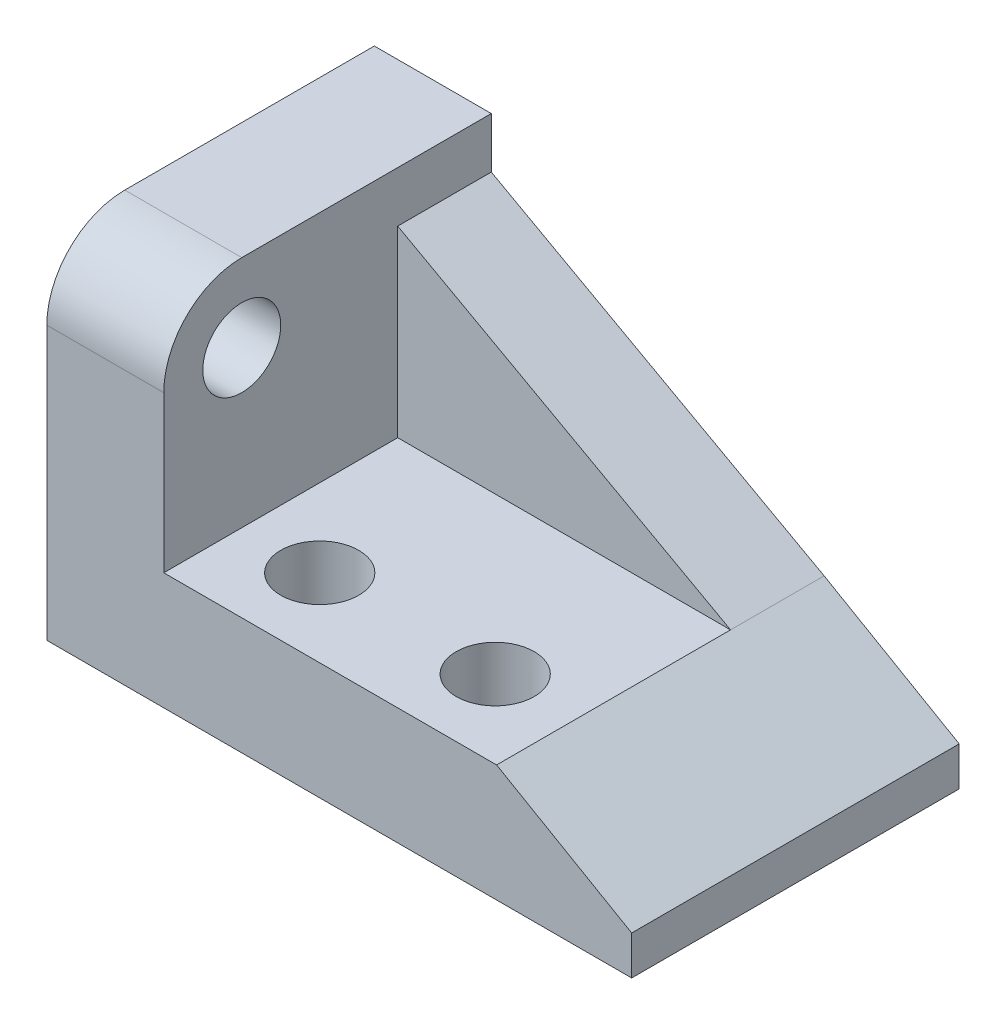
ISO-10303-21;
HEADER;
FILE_DESCRIPTION(('STEP AP214'),'2;1');
FILE_NAME('part.step','',(''),(''),'','','');
FILE_SCHEMA(('AUTOMOTIVE_DESIGN { 1 0 10303 214 1 1 1 1 }'));
ENDSEC;
DATA;
#1=APPLICATION_CONTEXT('core data for automotive mechanical design processes');
#2=APPLICATION_PROTOCOL_DEFINITION('international standard','automotive_design',2000,#1);
#3=PRODUCT_CONTEXT('',#1,'mechanical');
#4=PRODUCT('Part','Part','',(#3));
#5=PRODUCT_RELATED_PRODUCT_CATEGORY('part','',(#4));
#6=PRODUCT_DEFINITION_FORMATION('','',#4);
#7=PRODUCT_DEFINITION_CONTEXT('part definition',#1,'design');
#8=PRODUCT_DEFINITION('design','',#6,#7);
#9=PRODUCT_DEFINITION_SHAPE('','',#8);
#10=(LENGTH_UNIT() NAMED_UNIT(*) SI_UNIT(.MILLI.,.METRE.));
#11=(NAMED_UNIT(*) PLANE_ANGLE_UNIT() SI_UNIT($,.RADIAN.));
#12=(NAMED_UNIT(*) SI_UNIT($,.STERADIAN.) SOLID_ANGLE_UNIT());
#13=UNCERTAINTY_MEASURE_WITH_UNIT(LENGTH_MEASURE(1.E-05),#10,'distance_accuracy_value','');
#14=(GEOMETRIC_REPRESENTATION_CONTEXT(3) GLOBAL_UNCERTAINTY_ASSIGNED_CONTEXT((#13)) GLOBAL_UNIT_ASSIGNED_CONTEXT((#10,
#11,#12)) REPRESENTATION_CONTEXT('',''));
#15=CARTESIAN_POINT('',(0.,0.,0.));
#16=DIRECTION('',(0.,0.,1.));
#17=DIRECTION('',(1.,0.,0.));
#18=AXIS2_PLACEMENT_3D('',#15,#16,#17);
#19=CARTESIAN_POINT('',(40.3589838486223,30.,42.));
#20=DIRECTION('',(0.,-1.,0.));
#21=DIRECTION('',(1.,0.,0.));
#22=AXIS2_PLACEMENT_3D('',#19,#20,#21);
#23=PLANE('',#22);
#24=CARTESIAN_POINT('',(-25.,30.,22.));
#25=DIRECTION('',(0.,1.,0.));
#26=DIRECTION('',(-1.,0.,0.));
#27=AXIS2_PLACEMENT_3D('',#24,#25,#26);
#28=CIRCLE('',#27,10.);
#29=CARTESIAN_POINT('',(-35.,30.,22.));
#30=VERTEX_POINT('',#29);
#31=EDGE_CURVE('E214',#30,#30,#28,.T.);
#32=ORIENTED_EDGE('',*,*,#31,.F.);
#33=EDGE_LOOP('',(#32));
#34=FACE_BOUND('',#33,.T.);
#35=CARTESIAN_POINT('',(20.,30.,22.));
#36=DIRECTION('',(0.,1.,0.));
#37=DIRECTION('',(-1.,0.,0.));
#38=AXIS2_PLACEMENT_3D('',#35,#36,#37);
#39=CIRCLE('',#38,10.);
#40=CARTESIAN_POINT('',(9.99999999999999,30.,22.));
#41=VERTEX_POINT('',#40);
#42=EDGE_CURVE('E264',#41,#41,#39,.T.);
#43=ORIENTED_EDGE('',*,*,#42,.F.);
#44=EDGE_LOOP('',(#43));
#45=FACE_BOUND('',#44,.T.);
#46=DIRECTION('',(1.,0.,0.));
#47=VECTOR('',#46,1.);
#48=CARTESIAN_POINT('',(40.3589838486223,30.,-18.));
#49=LINE('',#48,#47);
#50=CARTESIAN_POINT('',(-45.,30.,-18.));
#51=VERTEX_POINT('',#50);
#52=CARTESIAN_POINT('',(40.3589838486223,30.,-18.));
#53=VERTEX_POINT('',#52);
#54=EDGE_CURVE('E153',#51,#53,#49,.T.);
#55=ORIENTED_EDGE('',*,*,#54,.F.);
#56=DIRECTION('',(0.,0.,-1.));
#57=VECTOR('',#56,1.);
#58=CARTESIAN_POINT('',(-45.,30.,42.));
#59=LINE('',#58,#57);
#60=CARTESIAN_POINT('',(-45.,30.,42.));
#61=VERTEX_POINT('',#60);
#62=EDGE_CURVE('E164',#61,#51,#59,.T.);
#63=ORIENTED_EDGE('',*,*,#62,.F.);
#64=DIRECTION('',(-1.,0.,0.));
#65=VECTOR('',#64,1.);
#66=CARTESIAN_POINT('',(40.3589838486223,30.,42.));
#67=LINE('',#66,#65);
#68=CARTESIAN_POINT('',(40.3589838486223,30.,42.));
#69=VERTEX_POINT('',#68);
#70=EDGE_CURVE('E144',#69,#61,#67,.T.);
#71=ORIENTED_EDGE('',*,*,#70,.F.);
#72=DIRECTION('',(0.,0.,-1.));
#73=VECTOR('',#72,1.);
#74=CARTESIAN_POINT('',(40.3589838486223,30.,42.));
#75=LINE('',#74,#73);
#76=EDGE_CURVE('E170',#69,#53,#75,.T.);
#77=ORIENTED_EDGE('',*,*,#76,.T.);
#78=EDGE_LOOP('',(#55,#63,#71,#77));
#79=FACE_BOUND('',#78,.T.);
#80=ADVANCED_FACE('F39',(#34,#45,#79),#23,.F.);
#81=CARTESIAN_POINT('',(-45.,90.,42.));
#82=DIRECTION('',(0.,-1.,0.));
#83=DIRECTION('',(0.,0.,-1.));
#84=AXIS2_PLACEMENT_3D('',#81,#82,#83);
#85=PLANE('',#84);
#86=DIRECTION('',(-1.,0.,0.));
#87=VECTOR('',#86,1.);
#88=CARTESIAN_POINT('',(-45.,90.,-42.));
#89=LINE('',#88,#87);
#90=CARTESIAN_POINT('',(-45.,90.,-42.));
#91=VERTEX_POINT('',#90);
#92=CARTESIAN_POINT('',(-75.,90.,-42.));
#93=VERTEX_POINT('',#92);
#94=EDGE_CURVE('E147',#91,#93,#89,.T.);
#95=ORIENTED_EDGE('',*,*,#94,.T.);
#96=DIRECTION('',(0.,0.,-1.));
#97=VECTOR('',#96,1.);
#98=CARTESIAN_POINT('',(-75.,90.,42.));
#99=LINE('',#98,#97);
#100=CARTESIAN_POINT('',(-75.,90.,22.));
#101=VERTEX_POINT('',#100);
#102=EDGE_CURVE('E135',#101,#93,#99,.T.);
#103=ORIENTED_EDGE('',*,*,#102,.F.);
#104=DIRECTION('',(-1.,0.,0.));
#105=VECTOR('',#104,1.);
#106=CARTESIAN_POINT('',(-45.,90.,22.));
#107=LINE('',#106,#105);
#108=CARTESIAN_POINT('',(-45.,90.,22.));
#109=VERTEX_POINT('',#108);
#110=EDGE_CURVE('E177',#101,#109,#107,.F.);
#111=ORIENTED_EDGE('',*,*,#110,.T.);
#112=DIRECTION('',(0.,0.,-1.));
#113=VECTOR('',#112,1.);
#114=CARTESIAN_POINT('',(-45.,90.,42.));
#115=LINE('',#114,#113);
#116=EDGE_CURVE('E149',#109,#91,#115,.T.);
#117=ORIENTED_EDGE('',*,*,#116,.T.);
#118=EDGE_LOOP('',(#95,#103,#111,#117));
#119=FACE_BOUND('',#118,.T.);
#120=ADVANCED_FACE('F189',(#119),#85,.F.);
#121=CARTESIAN_POINT('',(-75.,90.,42.));
#122=DIRECTION('',(1.,0.,0.));
#123=DIRECTION('',(0.,1.,0.));
#124=AXIS2_PLACEMENT_3D('',#121,#122,#123);
#125=PLANE('',#124);
#126=CARTESIAN_POINT('',(-75.,70.,22.));
#127=DIRECTION('',(1.,0.,0.));
#128=DIRECTION('',(0.,1.,0.));
#129=AXIS2_PLACEMENT_3D('',#126,#127,#128);
#130=CIRCLE('',#129,10.);
#131=CARTESIAN_POINT('',(-75.,80.,22.));
#132=VERTEX_POINT('',#131);
#133=EDGE_CURVE('E259',#132,#132,#130,.F.);
#134=ORIENTED_EDGE('',*,*,#133,.F.);
#135=EDGE_LOOP('',(#134));
#136=FACE_BOUND('',#135,.T.);
#137=DIRECTION('',(0.,-1.,0.));
#138=VECTOR('',#137,1.);
#139=CARTESIAN_POINT('',(-75.,90.,-42.));
#140=LINE('',#139,#138);
#141=CARTESIAN_POINT('',(-75.,0.,-42.));
#142=VERTEX_POINT('',#141);
#143=EDGE_CURVE('E129',#93,#142,#140,.T.);
#144=ORIENTED_EDGE('',*,*,#143,.T.);
#145=DIRECTION('',(0.,0.,-1.));
#146=VECTOR('',#145,1.);
#147=CARTESIAN_POINT('',(-75.,0.,42.));
#148=LINE('',#147,#146);
#149=CARTESIAN_POINT('',(-75.,0.,42.));
#150=VERTEX_POINT('',#149);
#151=EDGE_CURVE('E127',#150,#142,#148,.T.);
#152=ORIENTED_EDGE('',*,*,#151,.F.);
#153=DIRECTION('',(0.,-1.,0.));
#154=VECTOR('',#153,1.);
#155=CARTESIAN_POINT('',(-75.,90.,42.));
#156=LINE('',#155,#154);
#157=CARTESIAN_POINT('',(-75.,70.,42.));
#158=VERTEX_POINT('',#157);
#159=EDGE_CURVE('E114',#158,#150,#156,.T.);
#160=ORIENTED_EDGE('',*,*,#159,.F.);
#161=CARTESIAN_POINT('',(-75.,70.,22.));
#162=DIRECTION('',(1.,0.,0.));
#163=DIRECTION('',(0.,1.,0.));
#164=AXIS2_PLACEMENT_3D('',#161,#162,#163);
#165=CIRCLE('',#164,20.);
#166=EDGE_CURVE('E171',#158,#101,#165,.F.);
#167=ORIENTED_EDGE('',*,*,#166,.T.);
#168=ORIENTED_EDGE('',*,*,#102,.T.);
#169=EDGE_LOOP('',(#144,#152,#160,#167,#168));
#170=FACE_BOUND('',#169,.T.);
#171=ADVANCED_FACE('F130',(#136,#170),#125,.F.);
#172=CARTESIAN_POINT('',(-75.,0.,42.));
#173=DIRECTION('',(0.,1.,0.));
#174=DIRECTION('',(0.,0.,1.));
#175=AXIS2_PLACEMENT_3D('',#172,#173,#174);
#176=PLANE('',#175);
#177=CARTESIAN_POINT('',(-25.,0.,22.));
#178=DIRECTION('',(0.,1.,0.));
#179=DIRECTION('',(0.,0.,1.));
#180=AXIS2_PLACEMENT_3D('',#177,#178,#179);
#181=CIRCLE('',#180,10.);
#182=CARTESIAN_POINT('',(-25.,0.,32.));
#183=VERTEX_POINT('',#182);
#184=EDGE_CURVE('E207',#183,#183,#181,.F.);
#185=ORIENTED_EDGE('',*,*,#184,.F.);
#186=EDGE_LOOP('',(#185));
#187=FACE_BOUND('',#186,.T.);
#188=CARTESIAN_POINT('',(20.,0.,22.));
#189=DIRECTION('',(0.,1.,0.));
#190=DIRECTION('',(0.,0.,1.));
#191=AXIS2_PLACEMENT_3D('',#188,#189,#190);
#192=CIRCLE('',#191,10.);
#193=CARTESIAN_POINT('',(20.,0.,32.));
#194=VERTEX_POINT('',#193);
#195=EDGE_CURVE('E261',#194,#194,#192,.F.);
#196=ORIENTED_EDGE('',*,*,#195,.F.);
#197=EDGE_LOOP('',(#196));
#198=FACE_BOUND('',#197,.T.);
#199=DIRECTION('',(1.,0.,0.));
#200=VECTOR('',#199,1.);
#201=CARTESIAN_POINT('',(-75.,0.,-42.));
#202=LINE('',#201,#200);
#203=CARTESIAN_POINT('',(75.,0.,-42.));
#204=VERTEX_POINT('',#203);
#205=EDGE_CURVE('E154',#142,#204,#202,.T.);
#206=ORIENTED_EDGE('',*,*,#205,.T.);
#207=DIRECTION('',(0.,0.,-1.));
#208=VECTOR('',#207,1.);
#209=CARTESIAN_POINT('',(75.,0.,42.));
#210=LINE('',#209,#208);
#211=CARTESIAN_POINT('',(75.,0.,42.));
#212=VERTEX_POINT('',#211);
#213=EDGE_CURVE('E131',#212,#204,#210,.T.);
#214=ORIENTED_EDGE('',*,*,#213,.F.);
#215=DIRECTION('',(1.,0.,0.));
#216=VECTOR('',#215,1.);
#217=CARTESIAN_POINT('',(-75.,0.,42.));
#218=LINE('',#217,#216);
#219=EDGE_CURVE('E120',#150,#212,#218,.T.);
#220=ORIENTED_EDGE('',*,*,#219,.F.);
#221=ORIENTED_EDGE('',*,*,#151,.T.);
#222=EDGE_LOOP('',(#206,#214,#220,#221));
#223=FACE_BOUND('',#222,.T.);
#224=ADVANCED_FACE('F137',(#187,#198,#223),#176,.F.);
#225=CARTESIAN_POINT('',(75.,0.,42.));
#226=DIRECTION('',(-1.,0.,0.));
#227=DIRECTION('',(0.,-1.,0.));
#228=AXIS2_PLACEMENT_3D('',#225,#226,#227);
#229=PLANE('',#228);
#230=DIRECTION('',(0.,1.,0.));
#231=VECTOR('',#230,1.);
#232=CARTESIAN_POINT('',(75.,0.,-42.));
#233=LINE('',#232,#231);
#234=CARTESIAN_POINT('',(75.,10.,-42.));
#235=VERTEX_POINT('',#234);
#236=EDGE_CURVE('E160',#204,#235,#233,.T.);
#237=ORIENTED_EDGE('',*,*,#236,.T.);
#238=DIRECTION('',(0.,0.,-1.));
#239=VECTOR('',#238,1.);
#240=CARTESIAN_POINT('',(75.,10.,42.));
#241=LINE('',#240,#239);
#242=CARTESIAN_POINT('',(75.,10.,42.));
#243=VERTEX_POINT('',#242);
#244=EDGE_CURVE('E166',#243,#235,#241,.T.);
#245=ORIENTED_EDGE('',*,*,#244,.F.);
#246=DIRECTION('',(0.,1.,0.));
#247=VECTOR('',#246,1.);
#248=CARTESIAN_POINT('',(75.,0.,42.));
#249=LINE('',#248,#247);
#250=EDGE_CURVE('E138',#212,#243,#249,.T.);
#251=ORIENTED_EDGE('',*,*,#250,.F.);
#252=ORIENTED_EDGE('',*,*,#213,.T.);
#253=EDGE_LOOP('',(#237,#245,#251,#252));
#254=FACE_BOUND('',#253,.T.);
#255=ADVANCED_FACE('F197',(#254),#229,.F.);
#256=CARTESIAN_POINT('',(75.,10.,42.));
#257=DIRECTION('',(-0.499999999999998,-0.86602540378444,0.));
#258=DIRECTION('',(0.86602540378444,-0.499999999999998,0.));
#259=AXIS2_PLACEMENT_3D('',#256,#257,#258);
#260=PLANE('',#259);
#261=DIRECTION('',(0.,0.,-1.));
#262=VECTOR('',#261,1.);
#263=CARTESIAN_POINT('',(40.3589838486223,30.,42.));
#264=LINE('',#263,#262);
#265=CARTESIAN_POINT('',(40.3589838486223,30.,-42.));
#266=VERTEX_POINT('',#265);
#267=EDGE_CURVE('E53',#266,#53,#264,.F.);
#268=ORIENTED_EDGE('',*,*,#267,.T.);
#269=ORIENTED_EDGE('',*,*,#76,.F.);
#270=DIRECTION('',(-0.86602540378444,0.499999999999998,0.));
#271=VECTOR('',#270,1.);
#272=CARTESIAN_POINT('',(75.,10.,42.));
#273=LINE('',#272,#271);
#274=EDGE_CURVE('E136',#243,#69,#273,.T.);
#275=ORIENTED_EDGE('',*,*,#274,.F.);
#276=ORIENTED_EDGE('',*,*,#244,.T.);
#277=DIRECTION('',(-0.86602540378444,0.499999999999998,0.));
#278=VECTOR('',#277,1.);
#279=CARTESIAN_POINT('',(75.,10.,-42.));
#280=LINE('',#279,#278);
#281=EDGE_CURVE('E159',#235,#266,#280,.T.);
#282=ORIENTED_EDGE('',*,*,#281,.T.);
#283=EDGE_LOOP('',(#268,#269,#275,#276,#282));
#284=FACE_BOUND('',#283,.T.);
#285=ADVANCED_FACE('F200',(#284),#260,.F.);
#286=CARTESIAN_POINT('',(-45.,30.,42.));
#287=DIRECTION('',(-1.,0.,0.));
#288=DIRECTION('',(0.,0.,1.));
#289=AXIS2_PLACEMENT_3D('',#286,#287,#288);
#290=PLANE('',#289);
#291=CARTESIAN_POINT('',(-45.,70.,22.));
#292=DIRECTION('',(1.,0.,0.));
#293=DIRECTION('',(0.,0.,-1.));
#294=AXIS2_PLACEMENT_3D('',#291,#292,#293);
#295=CIRCLE('',#294,10.);
#296=CARTESIAN_POINT('',(-45.,70.,12.));
#297=VERTEX_POINT('',#296);
#298=EDGE_CURVE('E265',#297,#297,#295,.T.);
#299=ORIENTED_EDGE('',*,*,#298,.F.);
#300=EDGE_LOOP('',(#299));
#301=FACE_BOUND('',#300,.T.);
#302=DIRECTION('',(0.,-1.,0.));
#303=VECTOR('',#302,1.);
#304=CARTESIAN_POINT('',(-45.,30.,-18.));
#305=LINE('',#304,#303);
#306=CARTESIAN_POINT('',(-45.,77.,-18.));
#307=VERTEX_POINT('',#306);
#308=EDGE_CURVE('E11',#307,#51,#305,.T.);
#309=ORIENTED_EDGE('',*,*,#308,.F.);
#310=DIRECTION('',(0.,0.,1.));
#311=VECTOR('',#310,1.);
#312=CARTESIAN_POINT('',(-45.,77.,42.));
#313=LINE('',#312,#311);
#314=CARTESIAN_POINT('',(-45.,77.,-42.));
#315=VERTEX_POINT('',#314);
#316=EDGE_CURVE('E215',#307,#315,#313,.F.);
#317=ORIENTED_EDGE('',*,*,#316,.T.);
#318=DIRECTION('',(0.,1.,0.));
#319=VECTOR('',#318,1.);
#320=CARTESIAN_POINT('',(-45.,30.,-42.));
#321=LINE('',#320,#319);
#322=EDGE_CURVE('E123',#315,#91,#321,.T.);
#323=ORIENTED_EDGE('',*,*,#322,.T.);
#324=ORIENTED_EDGE('',*,*,#116,.F.);
#325=CARTESIAN_POINT('',(-45.,70.,22.));
#326=DIRECTION('',(-1.,0.,0.));
#327=DIRECTION('',(0.,0.,1.));
#328=AXIS2_PLACEMENT_3D('',#325,#326,#327);
#329=CIRCLE('',#328,20.);
#330=CARTESIAN_POINT('',(-45.,70.,42.));
#331=VERTEX_POINT('',#330);
#332=EDGE_CURVE('E50',#109,#331,#329,.F.);
#333=ORIENTED_EDGE('',*,*,#332,.T.);
#334=DIRECTION('',(0.,1.,0.));
#335=VECTOR('',#334,1.);
#336=CARTESIAN_POINT('',(-45.,30.,42.));
#337=LINE('',#336,#335);
#338=EDGE_CURVE('E150',#61,#331,#337,.T.);
#339=ORIENTED_EDGE('',*,*,#338,.F.);
#340=ORIENTED_EDGE('',*,*,#62,.T.);
#341=EDGE_LOOP('',(#309,#317,#323,#324,#333,#339,#340));
#342=FACE_BOUND('',#341,.T.);
#343=ADVANCED_FACE('F176',(#301,#342),#290,.F.);
#344=CARTESIAN_POINT('',(0.,0.,42.));
#345=DIRECTION('',(0.,0.,1.));
#346=DIRECTION('',(1.,0.,0.));
#347=AXIS2_PLACEMENT_3D('',#344,#345,#346);
#348=PLANE('',#347);
#349=ORIENTED_EDGE('',*,*,#338,.T.);
#350=DIRECTION('',(-1.,0.,0.));
#351=VECTOR('',#350,1.);
#352=CARTESIAN_POINT('',(-75.,70.,42.));
#353=LINE('',#352,#351);
#354=EDGE_CURVE('E122',#331,#158,#353,.T.);
#355=ORIENTED_EDGE('',*,*,#354,.T.);
#356=ORIENTED_EDGE('',*,*,#159,.T.);
#357=ORIENTED_EDGE('',*,*,#219,.T.);
#358=ORIENTED_EDGE('',*,*,#250,.T.);
#359=ORIENTED_EDGE('',*,*,#274,.T.);
#360=ORIENTED_EDGE('',*,*,#70,.T.);
#361=EDGE_LOOP('',(#349,#355,#356,#357,#358,#359,#360));
#362=FACE_BOUND('',#361,.T.);
#363=ADVANCED_FACE('F117',(#362),#348,.T.);
#364=CARTESIAN_POINT('',(0.,0.,-42.));
#365=DIRECTION('',(0.,0.,1.));
#366=DIRECTION('',(1.,0.,0.));
#367=AXIS2_PLACEMENT_3D('',#364,#365,#366);
#368=PLANE('',#367);
#369=ORIENTED_EDGE('',*,*,#322,.F.);
#370=DIRECTION('',(-0.875988049467589,0.482332807499105,0.));
#371=VECTOR('',#370,1.);
#372=CARTESIAN_POINT('',(40.3589838486223,30.,-42.));
#373=LINE('',#372,#371);
#374=EDGE_CURVE('E208',#266,#315,#373,.T.);
#375=ORIENTED_EDGE('',*,*,#374,.F.);
#376=ORIENTED_EDGE('',*,*,#281,.F.);
#377=ORIENTED_EDGE('',*,*,#236,.F.);
#378=ORIENTED_EDGE('',*,*,#205,.F.);
#379=ORIENTED_EDGE('',*,*,#143,.F.);
#380=ORIENTED_EDGE('',*,*,#94,.F.);
#381=EDGE_LOOP('',(#369,#375,#376,#377,#378,#379,#380));
#382=FACE_BOUND('',#381,.T.);
#383=ADVANCED_FACE('F192',(#382),#368,.F.);
#384=CARTESIAN_POINT('',(0.,70.,22.));
#385=DIRECTION('',(1.,0.,0.));
#386=DIRECTION('',(0.,0.,-1.));
#387=AXIS2_PLACEMENT_3D('',#384,#385,#386);
#388=CYLINDRICAL_SURFACE('',#387,20.);
#389=ORIENTED_EDGE('',*,*,#332,.F.);
#390=ORIENTED_EDGE('',*,*,#110,.F.);
#391=ORIENTED_EDGE('',*,*,#166,.F.);
#392=ORIENTED_EDGE('',*,*,#354,.F.);
#393=EDGE_LOOP('',(#389,#390,#391,#392));
#394=FACE_BOUND('',#393,.T.);
#395=ADVANCED_FACE('F41',(#394),#388,.T.);
#396=CARTESIAN_POINT('',(0.,45.,-18.));
#397=DIRECTION('',(0.,0.,-1.));
#398=DIRECTION('',(-1.,0.,0.));
#399=AXIS2_PLACEMENT_3D('',#396,#397,#398);
#400=PLANE('',#399);
#401=ORIENTED_EDGE('',*,*,#308,.T.);
#402=ORIENTED_EDGE('',*,*,#54,.T.);
#403=DIRECTION('',(-0.875988049467589,0.482332807499105,0.));
#404=VECTOR('',#403,1.);
#405=CARTESIAN_POINT('',(40.3589838486223,30.,-18.));
#406=LINE('',#405,#404);
#407=EDGE_CURVE('E206',#53,#307,#406,.T.);
#408=ORIENTED_EDGE('',*,*,#407,.T.);
#409=EDGE_LOOP('',(#401,#402,#408));
#410=FACE_BOUND('',#409,.T.);
#411=ADVANCED_FACE('F204',(#410),#400,.F.);
#412=CARTESIAN_POINT('',(40.3589838486223,30.,-42.));
#413=DIRECTION('',(-0.482332807499105,-0.875988049467589,0.));
#414=DIRECTION('',(-0.875988049467589,0.482332807499105,0.));
#415=AXIS2_PLACEMENT_3D('',#412,#413,#414);
#416=PLANE('',#415);
#417=ORIENTED_EDGE('',*,*,#267,.F.);
#418=ORIENTED_EDGE('',*,*,#374,.T.);
#419=ORIENTED_EDGE('',*,*,#316,.F.);
#420=ORIENTED_EDGE('',*,*,#407,.F.);
#421=EDGE_LOOP('',(#417,#418,#419,#420));
#422=FACE_BOUND('',#421,.T.);
#423=ADVANCED_FACE('F219',(#422),#416,.F.);
#424=CARTESIAN_POINT('',(20.,-0.00100000000000447,22.));
#425=DIRECTION('',(0.,1.,0.));
#426=DIRECTION('',(-1.,0.,0.));
#427=AXIS2_PLACEMENT_3D('',#424,#425,#426);
#428=CYLINDRICAL_SURFACE('',#427,10.);
#429=ORIENTED_EDGE('',*,*,#42,.T.);
#430=EDGE_LOOP('',(#429));
#431=FACE_BOUND('',#430,.T.);
#432=ORIENTED_EDGE('',*,*,#195,.T.);
#433=EDGE_LOOP('',(#432));
#434=FACE_BOUND('',#433,.T.);
#435=ADVANCED_FACE('F225',(#431,#434),#428,.F.);
#436=CARTESIAN_POINT('',(-25.,-0.00100000000000447,22.));
#437=DIRECTION('',(0.,1.,0.));
#438=DIRECTION('',(-1.,0.,0.));
#439=AXIS2_PLACEMENT_3D('',#436,#437,#438);
#440=CYLINDRICAL_SURFACE('',#439,10.);
#441=ORIENTED_EDGE('',*,*,#31,.T.);
#442=EDGE_LOOP('',(#441));
#443=FACE_BOUND('',#442,.T.);
#444=ORIENTED_EDGE('',*,*,#184,.T.);
#445=EDGE_LOOP('',(#444));
#446=FACE_BOUND('',#445,.T.);
#447=ADVANCED_FACE('F226',(#443,#446),#440,.F.);
#448=CARTESIAN_POINT('',(-75.001,70.,22.));
#449=DIRECTION('',(1.,0.,0.));
#450=DIRECTION('',(0.,0.,-1.));
#451=AXIS2_PLACEMENT_3D('',#448,#449,#450);
#452=CYLINDRICAL_SURFACE('',#451,10.);
#453=ORIENTED_EDGE('',*,*,#298,.T.);
#454=EDGE_LOOP('',(#453));
#455=FACE_BOUND('',#454,.T.);
#456=ORIENTED_EDGE('',*,*,#133,.T.);
#457=EDGE_LOOP('',(#456));
#458=FACE_BOUND('',#457,.T.);
#459=ADVANCED_FACE('F279',(#455,#458),#452,.F.);
#460=CLOSED_SHELL('',(#80,#120,#171,#224,#255,#285,#343,#363,#383,#395,#411,#423,#435,#447,#459));
#461=MANIFOLD_SOLID_BREP('B2',#460);
#462=ADVANCED_BREP_SHAPE_REPRESENTATION('',(#18,#461),#14);
#463=SHAPE_DEFINITION_REPRESENTATION(#9,#462);
ENDSEC;
END-ISO-10303-21;
